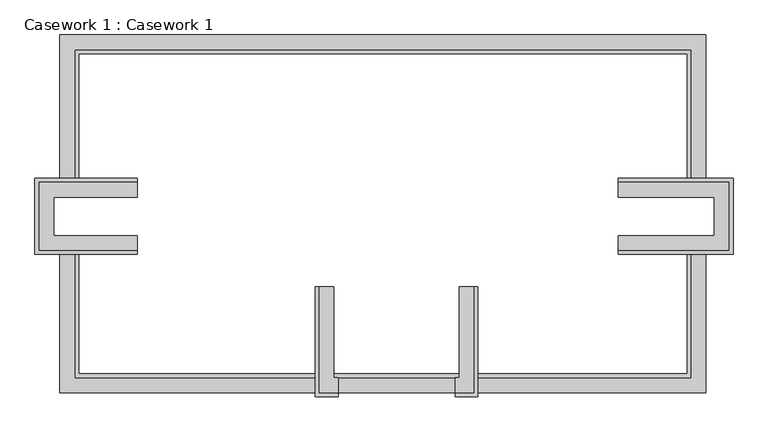
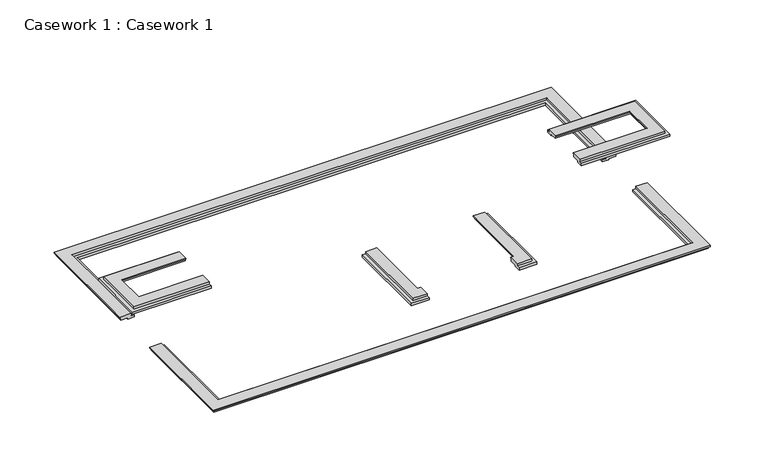
"""IFC4 building model written with IfcOpenShell, lengths in millimetres: furniture geometry, Casework 1 : Casework 1."""

from ifc_helpers import new_model, si_unit, origin, place, context, project, spatial, faceted_brep, source, transform, mapped, element, save


def casework_1_casework_1_4375437f(model_context):
    return source(origin(), model_context, "Body", "Brep", [
        faceted_brep([(8493.5830368, -13678.0592374, 7800.0), (8493.5830368, -12978.0592374, 7800.0), (8493.5830368, -12978.0592374, 7725.0), (8493.5830368, -13053.0592374, 7725.0), (8493.5830368, -13053.0592374, 7580.0), (8493.5830368, -13478.0592374, 7580.0), (8493.5830368, -13478.0592374, 7500.0), (8493.5830368, -13878.0592374, 7500.0), (8493.5830368, -13878.0592374, 7650.0), (8493.5830368, -13678.0592374, 7650.0), (9393.5830368, -13678.0592374, 7800.0), (9393.5830368, -13678.0592374, 7650.0), (9393.5830368, -8603.0592374, 7650.0), (9393.5830368, -8603.0592374, 7800.0), (9593.5830368, -13878.0592374, 7650.0), (9593.5830368, -13878.0592374, 7500.0), (9593.5830368, -8603.0592374, 7500.0), (9593.5830368, -8603.0592374, 7650.0), (9193.5830368, -13478.0592374, 7500.0), (9193.5830368, -13478.0592374, 7580.0), (9193.5830368, -8603.0592374, 7580.0), (9193.5830368, -8603.0592374, 7500.0), (8768.5830368, -13053.0592374, 7580.0), (8768.5830368, -13053.0592374, 7725.0), (8768.5830368, -8603.0592374, 7725.0), (8768.5830368, -8603.0592374, 7580.0), (8693.5830368, -12978.0592374, 7725.0), (8693.5830368, -12978.0592374, 7800.0), (8693.5830368, -8603.0592374, 7800.0), (8693.5830368, -8603.0592374, 7725.0)], [[[0, 1, 2, 3, 4, 5, 6, 7, 8, 9]], [[10, 11, 12, 13]], [[14, 15, 16, 17]], [[18, 19, 20, 21]], [[22, 23, 24, 25]], [[26, 27, 28, 29]], [[0, 9, 11, 10]], [[9, 8, 14, 17, 12, 11]], [[8, 7, 15, 14]], [[6, 18, 21, 16, 15, 7]], [[6, 5, 19, 18]], [[5, 4, 22, 25, 20, 19]], [[4, 3, 23, 22]], [[3, 2, 26, 29, 24, 23]], [[2, 1, 27, 26]], [[1, 0, 10, 13, 28, 27]], [[13, 12, 17, 16, 21, 20, 25, 24, 29, 28]]]),
        faceted_brep([(2893.5830368, -13678.0592374, 7800.0), (2893.5830368, -13678.0592374, 7650.0), (2893.5830368, -13878.0592374, 7650.0), (2893.5830368, -13878.0592374, 7500.0), (2893.5830368, -13478.0592374, 7500.0), (2893.5830368, -13478.0592374, 7580.0), (2893.5830368, -13053.0592374, 7580.0), (2893.5830368, -13053.0592374, 7725.0), (2893.5830368, -12978.0592374, 7725.0), (2893.5830368, -12978.0592374, 7800.0), (1993.5830368, -13678.0592374, 7650.0), (1993.5830368, -13678.0592374, 7800.0), (1993.5830368, -8603.0592374, 7800.0), (1993.5830368, -8603.0592374, 7650.0), (1793.5830368, -13878.0592374, 7500.0), (1793.5830368, -13878.0592374, 7650.0), (1793.5830368, -8603.0592374, 7650.0), (1793.5830368, -8603.0592374, 7500.0), (2193.5830368, -13478.0592374, 7580.0), (2193.5830368, -13478.0592374, 7500.0), (2193.5830368, -8603.0592374, 7500.0), (2193.5830368, -8603.0592374, 7580.0), (2618.5830368, -13053.0592374, 7725.0), (2618.5830368, -13053.0592374, 7580.0), (2618.5830368, -8603.0592374, 7580.0), (2618.5830368, -8603.0592374, 7725.0), (2693.5830368, -12978.0592374, 7800.0), (2693.5830368, -12978.0592374, 7725.0), (2693.5830368, -8603.0592374, 7725.0), (2693.5830368, -8603.0592374, 7800.0)], [[[0, 1, 2, 3, 4, 5, 6, 7, 8, 9]], [[10, 11, 12, 13]], [[14, 15, 16, 17]], [[18, 19, 20, 21]], [[22, 23, 24, 25]], [[26, 27, 28, 29]], [[1, 0, 11, 10]], [[3, 2, 15, 14]], [[5, 4, 19, 18]], [[7, 6, 23, 22]], [[9, 8, 27, 26]], [[12, 29, 28, 25, 24, 21, 20, 17, 16, 13]], [[2, 1, 10, 13, 16, 15]], [[3, 14, 17, 20, 19, 4]], [[6, 5, 18, 21, 24, 23]], [[8, 7, 22, 25, 28, 27]], [[0, 9, 26, 29, 12, 11]]]),
        faceted_brep([(16306.0830368, -6865.5592374, 7800.0), (16306.0830368, -6165.5592374, 7800.0), (16306.0830368, -6165.5592374, 7725.0), (16306.0830368, -6240.5592374, 7725.0), (16306.0830368, -6240.5592374, 7580.0), (16306.0830368, -6665.5592374, 7580.0), (16306.0830368, -6665.5592374, 7500.0), (16306.0830368, -7065.5592374, 7500.0), (16306.0830368, -7065.5592374, 7650.0), (16306.0830368, -6865.5592374, 7650.0), (21606.0830368, -3615.5592374, 7800.0), (21606.0830368, -3615.5592374, 7650.0), (16306.0830368, -3615.5592374, 7650.0), (16306.0830368, -3615.5592374, 7800.0), (21806.0830368, -3415.5592374, 7650.0), (21806.0830368, -3415.5592374, 7500.0), (16306.0830368, -3415.5592374, 7500.0), (16306.0830368, -3415.5592374, 7650.0), (21406.0830368, -3815.5592374, 7500.0), (21406.0830368, -3815.5592374, 7580.0), (16306.0830368, -3815.5592374, 7580.0), (16306.0830368, -3815.5592374, 7500.0), (20981.0830368, -4240.5592374, 7580.0), (20981.0830368, -4240.5592374, 7725.0), (16306.0830368, -4240.5592374, 7725.0), (16306.0830368, -4240.5592374, 7580.0), (20906.0830368, -4315.5592374, 7725.0), (20906.0830368, -4315.5592374, 7800.0), (16306.0830368, -4315.5592374, 7800.0), (16306.0830368, -4315.5592374, 7725.0), (21606.0830368, -6865.5592374, 7800.0), (21606.0830368, -6865.5592374, 7650.0), (21806.0830368, -7065.5592374, 7650.0), (21806.0830368, -7065.5592374, 7500.0), (21406.0830368, -6665.5592374, 7500.0), (21406.0830368, -6665.5592374, 7580.0), (20981.0830368, -6240.5592374, 7580.0), (20981.0830368, -6240.5592374, 7725.0), (20906.0830368, -6165.5592374, 7725.0), (20906.0830368, -6165.5592374, 7800.0)], [[[0, 1, 2, 3, 4, 5, 6, 7, 8, 9]], [[10, 11, 12, 13]], [[14, 15, 16, 17]], [[18, 19, 20, 21]], [[22, 23, 24, 25]], [[26, 27, 28, 29]], [[30, 31, 11, 10]], [[32, 33, 15, 14]], [[34, 35, 19, 18]], [[36, 37, 23, 22]], [[38, 39, 27, 26]], [[13, 12, 17, 16, 21, 20, 25, 24, 29, 28]], [[0, 9, 31, 30]], [[9, 8, 32, 14, 17, 12, 11, 31]], [[8, 7, 33, 32]], [[6, 34, 18, 21, 16, 15, 33, 7]], [[6, 5, 35, 34]], [[5, 4, 36, 22, 25, 20, 19, 35]], [[4, 3, 37, 36]], [[3, 2, 38, 26, 29, 24, 23, 37]], [[2, 1, 39, 38]], [[1, 0, 30, 10, 13, 28, 27, 39]]]),
        faceted_brep([(-6716.8860603, -6865.5592374, 7800.0), (-6716.8860603, -6865.5592374, 7650.0), (-6716.8860603, -7065.5592374, 7650.0), (-6716.8860603, -7065.5592374, 7500.0), (-6716.8860603, -6665.5592374, 7500.0), (-6716.8860603, -6665.5592374, 7580.0), (-6716.8860603, -6240.5592374, 7580.0), (-6716.8860603, -6240.5592374, 7725.0), (-6716.8860603, -6165.5592374, 7725.0), (-6716.8860603, -6165.5592374, 7800.0), (-11418.9169632, -3615.5592374, 7650.0), (-11418.9169632, -3615.5592374, 7800.0), (-6716.8860603, -3615.5592374, 7800.0), (-6716.8860603, -3615.5592374, 7650.0), (-11618.9169632, -3415.5592374, 7500.0), (-11618.9169632, -3415.5592374, 7650.0), (-6716.8860603, -3415.5592374, 7650.0), (-6716.8860603, -3415.5592374, 7500.0), (-11218.9169632, -3815.5592374, 7580.0), (-11218.9169632, -3815.5592374, 7500.0), (-6716.8860603, -3815.5592374, 7500.0), (-6716.8860603, -3815.5592374, 7580.0), (-10793.9169632, -4240.5592374, 7725.0), (-10793.9169632, -4240.5592374, 7580.0), (-6716.8860603, -4240.5592374, 7580.0), (-6716.8860603, -4240.5592374, 7725.0), (-10718.9169632, -4315.5592374, 7800.0), (-10718.9169632, -4315.5592374, 7725.0), (-6716.8860603, -4315.5592374, 7725.0), (-6716.8860603, -4315.5592374, 7800.0), (-11418.9169632, -6865.5592374, 7650.0), (-11418.9169632, -6865.5592374, 7800.0), (-11618.9169632, -7065.5592374, 7500.0), (-11618.9169632, -7065.5592374, 7650.0), (-11218.9169632, -6665.5592374, 7580.0), (-11218.9169632, -6665.5592374, 7500.0), (-10793.9169632, -6240.5592374, 7725.0), (-10793.9169632, -6240.5592374, 7580.0), (-10718.9169632, -6165.5592374, 7800.0), (-10718.9169632, -6165.5592374, 7725.0)], [[[0, 1, 2, 3, 4, 5, 6, 7, 8, 9]], [[10, 11, 12, 13]], [[14, 15, 16, 17]], [[18, 19, 20, 21]], [[22, 23, 24, 25]], [[26, 27, 28, 29]], [[30, 31, 11, 10]], [[32, 33, 15, 14]], [[34, 35, 19, 18]], [[36, 37, 23, 22]], [[38, 39, 27, 26]], [[12, 29, 28, 25, 24, 21, 20, 17, 16, 13]], [[1, 0, 31, 30]], [[2, 1, 30, 10, 13, 16, 15, 33]], [[3, 2, 33, 32]], [[3, 32, 14, 17, 20, 19, 35, 4]], [[5, 4, 35, 34]], [[6, 5, 34, 18, 21, 24, 23, 37]], [[7, 6, 37, 36]], [[8, 7, 36, 22, 25, 28, 27, 39]], [[9, 8, 39, 38]], [[0, 9, 38, 26, 29, 12, 11, 31]]]),
        faceted_brep([(-9718.9169632, -3615.5592374, 4800.0), (-10418.9169632, -3615.5592374, 4800.0), (-10418.9169632, -3615.5592374, 4725.0), (-10343.9169632, -3615.5592374, 4725.0), (-10343.9169632, -3615.5592374, 4580.0), (-9918.9169632, -3615.5592374, 4580.0), (-9918.9169632, -3615.5592374, 4500.0), (-9518.9169632, -3615.5592374, 4500.0), (-9518.9169632, -3615.5592374, 4650.0), (-9718.9169632, -3615.5592374, 4650.0), (-9718.9169632, 2746.9407626, 4650.0), (-9718.9169632, 2746.9407626, 4800.0), (-9518.9169632, 2546.9407626, 4650.0), (19606.0830368, 2546.9407626, 4650.0), (19606.0830368, -3615.5592374, 4650.0), (19806.0830368, -3615.5592374, 4650.0), (19806.0830368, 2746.9407626, 4650.0), (-9518.9169632, 2546.9407626, 4500.0), (-9918.9169632, 2946.9407626, 4500.0), (20006.0830368, 2946.9407626, 4500.0), (20006.0830368, -3615.5592374, 4500.0), (19606.0830368, -3615.5592374, 4500.0), (19606.0830368, 2546.9407626, 4500.0), (-9918.9169632, 2946.9407626, 4580.0), (-10343.9169632, 3371.9407626, 4580.0), (20431.0830368, 3371.9407626, 4580.0), (20431.0830368, -3615.5592374, 4580.0), (20006.0830368, -3615.5592374, 4580.0), (20006.0830368, 2946.9407626, 4580.0), (-10343.9169632, 3371.9407626, 4725.0), (-10418.9169632, 3446.9407626, 4725.0), (20506.0830368, 3446.9407626, 4725.0), (20506.0830368, -3615.5592374, 4725.0), (20431.0830368, -3615.5592374, 4725.0), (20431.0830368, 3371.9407626, 4725.0), (-10418.9169632, 3446.9407626, 4800.0), (19806.0830368, 2746.9407626, 4800.0), (19806.0830368, -3615.5592374, 4800.0), (20506.0830368, -3615.5592374, 4800.0), (20506.0830368, 3446.9407626, 4800.0)], [[[0, 1, 2, 3, 4, 5, 6, 7, 8, 9]], [[0, 9, 10, 11]], [[9, 8, 12, 13, 14, 15, 16, 10]], [[8, 7, 17, 12]], [[6, 18, 19, 20, 21, 22, 17, 7]], [[6, 5, 23, 18]], [[5, 4, 24, 25, 26, 27, 28, 23]], [[4, 3, 29, 24]], [[3, 2, 30, 31, 32, 33, 34, 29]], [[2, 1, 35, 30]], [[1, 0, 11, 36, 37, 38, 39, 35]], [[11, 10, 16, 36]], [[12, 17, 22, 13]], [[18, 23, 28, 19]], [[24, 29, 34, 25]], [[30, 35, 39, 31]], [[37, 15, 14, 21, 20, 27, 26, 33, 32, 38]], [[36, 16, 15, 37]], [[13, 22, 21, 14]], [[19, 28, 27, 20]], [[25, 34, 33, 26]], [[31, 39, 38, 32]]]),
        faceted_brep([(-9718.9169632, -6865.5592374, 4800.0), (-9718.9169632, -6865.5592374, 4650.0), (-9518.9169632, -6865.5592374, 4650.0), (-9518.9169632, -6865.5592374, 4500.0), (-9918.9169632, -6865.5592374, 4500.0), (-9918.9169632, -6865.5592374, 4580.0), (-10343.9169632, -6865.5592374, 4580.0), (-10343.9169632, -6865.5592374, 4725.0), (-10418.9169632, -6865.5592374, 4725.0), (-10418.9169632, -6865.5592374, 4800.0), (-9718.9169632, -12978.0592374, 4800.0), (-9718.9169632, -12978.0592374, 4650.0), (19806.0830368, -12978.0592374, 4650.0), (19806.0830368, -6865.5592374, 4650.0), (19606.0830368, -6865.5592374, 4650.0), (19606.0830368, -12778.0592374, 4650.0), (-9518.9169632, -12778.0592374, 4650.0), (-9518.9169632, -12778.0592374, 4500.0), (19606.0830368, -12778.0592374, 4500.0), (19606.0830368, -6865.5592374, 4500.0), (20006.0830368, -6865.5592374, 4500.0), (20006.0830368, -13178.0592374, 4500.0), (-9918.9169632, -13178.0592374, 4500.0), (-9918.9169632, -13178.0592374, 4580.0), (20006.0830368, -13178.0592374, 4580.0), (20006.0830368, -6865.5592374, 4580.0), (20431.0830368, -6865.5592374, 4580.0), (20431.0830368, -13603.0592374, 4580.0), (-10343.9169632, -13603.0592374, 4580.0), (-10343.9169632, -13603.0592374, 4725.0), (20431.0830368, -13603.0592374, 4725.0), (20431.0830368, -6865.5592374, 4725.0), (20506.0830368, -6865.5592374, 4725.0), (20506.0830368, -13678.0592374, 4725.0), (-10418.9169632, -13678.0592374, 4725.0), (-10418.9169632, -13678.0592374, 4800.0), (20506.0830368, -13678.0592374, 4800.0), (20506.0830368, -6865.5592374, 4800.0), (19806.0830368, -6865.5592374, 4800.0), (19806.0830368, -12978.0592374, 4800.0)], [[[0, 1, 2, 3, 4, 5, 6, 7, 8, 9]], [[1, 0, 10, 11]], [[2, 1, 11, 12, 13, 14, 15, 16]], [[3, 2, 16, 17]], [[3, 17, 18, 19, 20, 21, 22, 4]], [[5, 4, 22, 23]], [[6, 5, 23, 24, 25, 26, 27, 28]], [[7, 6, 28, 29]], [[8, 7, 29, 30, 31, 32, 33, 34]], [[9, 8, 34, 35]], [[0, 9, 35, 36, 37, 38, 39, 10]], [[11, 10, 39, 12]], [[17, 16, 15, 18]], [[23, 22, 21, 24]], [[29, 28, 27, 30]], [[35, 34, 33, 36]], [[38, 37, 32, 31, 26, 25, 20, 19, 14, 13]], [[12, 39, 38, 13]], [[18, 15, 14, 19]], [[24, 21, 20, 25]], [[30, 27, 26, 31]], [[36, 33, 32, 37]]]),
    ])


if __name__ == "__main__":
    model = new_model("IFC4")
    model_context = context("Model", 3, world=origin())
    ifc_project = project(units=[si_unit("LENGTHUNIT", "METRE", prefix="MILLI")], contexts=[model_context])
    site = spatial("IfcSite", under=ifc_project)
    building = spatial("IfcBuilding", under=site)
    placement = place(None, origin())
    casework_1_casework_1_shape = casework_1_casework_1_4375437f(model_context)
    element("IfcFurniture", 1, ObjectType="Casework 1 : Casework 1", at=placement, inside=building, context=model_context, shape_type="MappedRepresentation", body=[
        mapped(casework_1_casework_1_shape, transform((0.0, 0.0, 0.0), x_axis=(1.0, 0.0, 0.0), y_axis=(0.0, 1.0, 0.0), z_axis=(0.0, 0.0, 1.0))),
    ])
    save(model, "model.ifc")
